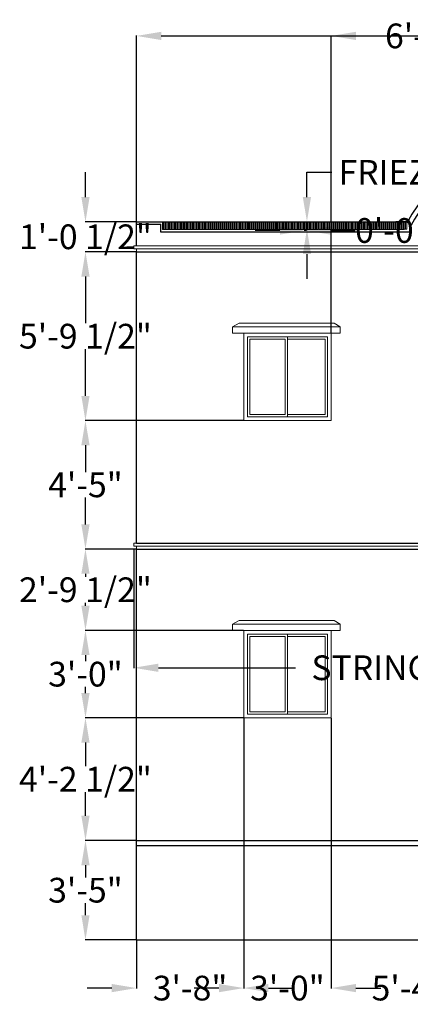
# Model space of a CAD drawing. Units: inches. Extents: x 2393 to 3270, y 740 to 1442.
# Tile 2 of 5: x 2393 to 2554, y 1031 to 1436. Entities that reach past the tile are written whole.
import ezdxf

# ---------------------------------------------------------------- set-up
doc = ezdxf.new("R2010")
doc.units = ezdxf.units.IN
doc.header["$MEASUREMENT"] = 0
for name, color, linetype, lineweight in [('A-ANNO-DIMS', 2, 'Continuous', 18), ('A-ELEV', 7, 'Continuous', 30), ('A-ELEV-TRIM', 8, 'Continuous', 13), ('A-GLAZ', 4, 'Continuous', 18), ('A-ROOF', 7, 'Continuous', 25)]:
    doc.layers.add(name, color=color, linetype=linetype, lineweight=lineweight)
doc.styles.get("Standard").update_dxf_attribs({"font": 'arial.ttf'})
doc.dimstyles.get("Standard").update_dxf_attribs({"dimtxt": 10.18, "dimasz": 10.18, "dimexe": 0.18, "dimexo": 0.0625, "dimgap": 0.09, "dimtad": 0, "dimtih": 1, "dimtoh": 1, "dimdec": 0, "dimzin": 0, "dimdsep": 46, "dimlunit": 3, "dimtxsty": 'Standard', "dimcen": 0.09, "dimadec": 0, "dimazin": 0, "dimtfac": 1, "dimtdec": 0, "dimtofl": 0, "dimtmove": 0, "dimatfit": 3, "dimfxl": 1, "dimtolj": 1, "dimtzin": 0, "dimarcsym": 0})

# ---------------------------------------------------------------- blocks, each defined once
blk = doc.blocks.new('*U4')
for p, q in [((1.5, 1.5), (1.5, 34.5)), ((1.5, 34.5), (18, 34.5)), ((18, 1.5), (18, 34.5)), ((18, 34.5), (34.5, 34.5)), ((34.5, 34.5), (34.5, 1.5)), ((18, 1.5), (1.5, 1.5)), ((34.5, 1.5), (18, 1.5))]:
    blk.add_line(p, q)
blk.add_lwpolyline([(0, 0), (0, 36), (36, 36), (36, 0)], close=True)
for points in [[(17, 33.5), (17, 2.5), (2.5, 2.5), (2.5, 33.5), (17, 33.5)], [(18, 33.5), (33.5, 33.5), (33.5, 2.5), (18, 2.5)]]:
    blk.add_lwpolyline(points)
blk = doc.blocks.new('WIN-HEAD-HOOD-ELEV')
for p, q in [((0, 2.55), (2.7, 4.11)), ((2.7, 4.11), (41.79, 4.11)), ((41.79, 4.11), (44.29, 2.55)), ((0, 0), (0, 2.55)), ((0, 2.55), (44.29, 2.55)), ((0, 0), (4.55, 0)), ((44.29, 0), (40.55, 0)), ((44.29, 2.55), (44.29, 0))]:
    blk.add_line(p, q)
blk = doc.blocks.new('FACADE-STRING-COURSE')
for p, q in [((0.49, 2.4), (0, 2.4)), ((0, 2.4), (0, 1.23)), ((0, 1.23), (1.17, 1.23)), ((0.49, 2.4), (325.84, 2.4)), ((325.84, 1.23), (325.17, 1.23)), ((325.84, 2.4), (325.84, 1.23))]:
    blk.add_line(p, q)
blk.add_lwpolyline([(1.17, 0), (325.17, 0), (325.17, 1.23), (1.17, 1.23)], close=True)
blk = doc.blocks.new('PARAPET-FRIEZE-MODULE')
blk.add_lwpolyline([(0, 3.12), (0.5, 3.12), (0.5, 0), (0, 0)], close=True)
blk = doc.blocks.new('*D38')
at = {"layer": 'A-ANNO-DIMS', "color": 0, "lineweight": -2, "transparency": 16777216}
for p, q in [((2511.53, 1363.37), (2511.53, 1373.55)), ((2511.53, 1373.55), (2521.71, 1373.55)), ((2511.12, 1353.19), (2511.71, 1353.19)), ((2511.12, 1350.06), (2511.71, 1350.06)), ((2511.53, 1339.88), (2511.53, 1329.7))]:
    blk.add_line(p, q, dxfattribs=at)
at = {"layer": 'A-ANNO-DIMS', "color": 0, "transparency": 16777216}
for points in [[(2509.83, 1363.37), (2513.22, 1363.37), (2511.53, 1353.19)], [(2509.83, 1339.88), (2513.22, 1339.88), (2511.53, 1350.06)]]:
    blk.add_solid(points, dxfattribs=at)
at = {"layer": 'Defpoints', "color": 0, "transparency": 16777216}
for p in [(2511.06, 1353.19), (2511.06, 1350.06), (2511.53, 1353.19)]:
    blk.add_point(p, dxfattribs=at)
at = {"layer": 'A-ANNO-DIMS', "color": 0, "transparency": 16777216, "insert": (2579.79, 1373.55), "char_height": 10.18, "attachment_point": 5}
blk.add_mtext('\\A1;FRIEZE 0\'-3" TYP.', dxfattribs=at)
blk = doc.blocks.new('*D39')
at = {"layer": 'A-ANNO-DIMS', "color": 0, "lineweight": -2, "transparency": 16777216}
for p, q in [((2500.38, 1349.6), (2490.2, 1349.6)), ((2510.56, 1350), (2510.56, 1349.42)), ((2511.06, 1350), (2511.06, 1349.42)), ((2521.24, 1349.6), (2531.42, 1349.6))]:
    blk.add_line(p, q, dxfattribs=at)
at = {"layer": 'A-ANNO-DIMS', "color": 0, "transparency": 16777216}
for points in [[(2500.38, 1351.29), (2500.38, 1347.9), (2510.56, 1349.6)], [(2521.24, 1351.29), (2521.24, 1347.9), (2511.06, 1349.6)]]:
    blk.add_solid(points, dxfattribs=at)
at = {"layer": 'Defpoints', "color": 0, "transparency": 16777216}
for p in [(2510.56, 1350.06), (2511.06, 1350.06), (2511.06, 1349.6)]:
    blk.add_point(p, dxfattribs=at)
at = {"layer": 'A-ANNO-DIMS', "color": 0, "transparency": 16777216, "insert": (2574.39, 1349.6), "char_height": 10.18, "attachment_point": 5}
blk.add_mtext('\\A1;0\'-0 1/2" TYP.', dxfattribs=at)
blk = doc.blocks.new('*D40')
at = {"layer": 'A-ANNO-DIMS', "color": 0, "lineweight": -2, "transparency": 16777216}
for p, q in [((2440.26, 1218.37), (2440.26, 1169.38)), ((2766.1, 1218.37), (2766.1, 1169.38)), ((2450.44, 1169.56), (2506.89, 1169.56)), ((2755.92, 1169.56), (2699.46, 1169.56))]:
    blk.add_line(p, q, dxfattribs=at)
at = {"layer": 'A-ANNO-DIMS', "color": 0, "transparency": 16777216}
for points in [[(2450.44, 1171.25), (2450.44, 1167.86), (2440.26, 1169.56)], [(2755.92, 1171.25), (2755.92, 1167.86), (2766.1, 1169.56)]]:
    blk.add_solid(points, dxfattribs=at)
at = {"layer": 'Defpoints', "color": 0, "transparency": 16777216}
for p in [(2440.26, 1218.43), (2766.1, 1218.43), (2766.1, 1169.56)]:
    blk.add_point(p, dxfattribs=at)
at = {"layer": 'A-ANNO-DIMS', "color": 0, "transparency": 16777216, "insert": (2603.18, 1169.56), "char_height": 10.18, "attachment_point": 5}
blk.add_mtext('\\A1;STRING COURSE 27\'-2" TYP.', dxfattribs=at)
blk = doc.blocks.new('*D57')
at = {"layer": 'A-ANNO-DIMS', "color": 0, "lineweight": -2, "transparency": 16777216}
for p, q in [((2441.43, 1353.25), (2441.43, 1429.9)), ((2451.61, 1429.72), (2585.76, 1429.72)), ((2755.25, 1429.72), (2621.09, 1429.72)), ((2765.43, 1353.25), (2765.43, 1429.9))]:
    blk.add_line(p, q, dxfattribs=at)
at = {"layer": 'A-ANNO-DIMS', "color": 0, "transparency": 16777216}
for points in [[(2451.61, 1431.41), (2451.61, 1428.02), (2441.43, 1429.72)], [(2755.25, 1431.41), (2755.25, 1428.02), (2765.43, 1429.72)]]:
    blk.add_solid(points, dxfattribs=at)
at = {"layer": 'Defpoints', "color": 0, "transparency": 16777216}
for p in [(2765.43, 1429.72), (2441.43, 1353.19), (2765.43, 1353.19)]:
    blk.add_point(p, dxfattribs=at)
at = {"layer": 'A-ANNO-DIMS', "color": 0, "transparency": 16777216, "insert": (2603.43, 1429.72), "char_height": 10.18, "attachment_point": 5}
blk.add_mtext('\\A1;27\'-0"', dxfattribs=at)
blk = doc.blocks.new('*D59')
at = {"layer": 'A-ANNO-DIMS', "color": 0, "lineweight": -2, "transparency": 16777216}
for p, q in [((2441.36, 1098.43), (2420.24, 1098.43)), ((2420.42, 1088.25), (2420.42, 1083.26)), ((2420.42, 1067.68), (2420.42, 1072.68)), ((2441.36, 1057.5), (2420.24, 1057.5))]:
    blk.add_line(p, q, dxfattribs=at)
at = {"layer": 'A-ANNO-DIMS', "color": 0, "transparency": 16777216}
for points in [[(2418.73, 1088.25), (2422.12, 1088.25), (2420.42, 1098.43)], [(2418.73, 1067.68), (2422.12, 1067.68), (2420.42, 1057.5)]]:
    blk.add_solid(points, dxfattribs=at)
at = {"layer": 'Defpoints', "color": 0, "transparency": 16777216}
for p in [(2420.42, 1098.43), (2441.43, 1098.43), (2441.43, 1057.5)]:
    blk.add_point(p, dxfattribs=at)
at = {"layer": 'A-ANNO-DIMS', "color": 0, "transparency": 16777216, "insert": (2420.42, 1077.97), "char_height": 10.18, "attachment_point": 5}
blk.add_mtext('\\A1;3\'-5"', dxfattribs=at)
blk = doc.blocks.new('*D60')
at = {"layer": 'A-ANNO-DIMS', "color": 0, "lineweight": -2, "transparency": 16777216}
for p, q in [((2485.45, 1148.93), (2420.24, 1148.93)), ((2420.42, 1138.75), (2420.42, 1129.04)), ((2420.42, 1108.61), (2420.42, 1118.33)), ((2441.36, 1098.43), (2420.24, 1098.43))]:
    blk.add_line(p, q, dxfattribs=at)
at = {"layer": 'A-ANNO-DIMS', "color": 0, "transparency": 16777216}
for points in [[(2418.73, 1138.75), (2422.12, 1138.75), (2420.42, 1148.93)], [(2418.73, 1108.61), (2422.12, 1108.61), (2420.42, 1098.43)]]:
    blk.add_solid(points, dxfattribs=at)
at = {"layer": 'Defpoints', "color": 0, "transparency": 16777216}
for p in [(2420.42, 1148.93), (2485.51, 1148.93), (2441.43, 1098.43)]:
    blk.add_point(p, dxfattribs=at)
at = {"layer": 'A-ANNO-DIMS', "color": 0, "transparency": 16777216, "insert": (2420.42, 1123.68), "char_height": 10.18, "attachment_point": 5}
blk.add_mtext('\\A1;4\'-2 1/2"', dxfattribs=at)
blk = doc.blocks.new('*D61')
at = {"layer": 'A-ANNO-DIMS', "color": 0, "lineweight": -2, "transparency": 16777216}
for p, q in [((2485.45, 1184.93), (2420.24, 1184.93)), ((2420.42, 1174.75), (2420.42, 1172.22)), ((2420.42, 1159.11), (2420.42, 1161.64)), ((2485.45, 1148.93), (2420.24, 1148.93))]:
    blk.add_line(p, q, dxfattribs=at)
at = {"layer": 'A-ANNO-DIMS', "color": 0, "transparency": 16777216}
for points in [[(2418.73, 1174.75), (2422.12, 1174.75), (2420.42, 1184.93)], [(2418.73, 1159.11), (2422.12, 1159.11), (2420.42, 1148.93)]]:
    blk.add_solid(points, dxfattribs=at)
at = {"layer": 'Defpoints', "color": 0, "transparency": 16777216}
for p in [(2420.42, 1184.93), (2485.51, 1184.93), (2485.51, 1148.93)]:
    blk.add_point(p, dxfattribs=at)
at = {"layer": 'A-ANNO-DIMS', "color": 0, "transparency": 16777216, "insert": (2420.42, 1166.93), "char_height": 10.18, "attachment_point": 5}
blk.add_mtext('\\A1;3\'-0"', dxfattribs=at)
blk = doc.blocks.new('*D62')
at = {"layer": 'A-ANNO-DIMS', "color": 0, "lineweight": -2, "transparency": 16777216}
for p, q in [((2441.36, 1218.43), (2420.24, 1218.43)), ((2420.42, 1208.25), (2420.42, 1207.04)), ((2420.42, 1195.11), (2420.42, 1196.33)), ((2485.45, 1184.93), (2420.24, 1184.93))]:
    blk.add_line(p, q, dxfattribs=at)
at = {"layer": 'A-ANNO-DIMS', "color": 0, "transparency": 16777216}
for points in [[(2418.73, 1208.25), (2422.12, 1208.25), (2420.42, 1218.43)], [(2418.73, 1195.11), (2422.12, 1195.11), (2420.42, 1184.93)]]:
    blk.add_solid(points, dxfattribs=at)
at = {"layer": 'Defpoints', "color": 0, "transparency": 16777216}
for p in [(2420.42, 1218.43), (2441.43, 1218.43), (2485.51, 1184.93)]:
    blk.add_point(p, dxfattribs=at)
at = {"layer": 'A-ANNO-DIMS', "color": 0, "transparency": 16777216, "insert": (2420.42, 1201.68), "char_height": 10.18, "attachment_point": 5}
blk.add_mtext('\\A1;2\'-9 1/2"', dxfattribs=at)
blk = doc.blocks.new('*D63')
at = {"layer": 'A-ANNO-DIMS', "color": 0, "lineweight": -2, "transparency": 16777216}
for p, q in [((2485.45, 1271.33), (2420.24, 1271.33)), ((2420.42, 1261.15), (2420.42, 1250.15)), ((2420.42, 1228.61), (2420.42, 1239.61)), ((2441.36, 1218.43), (2420.24, 1218.43))]:
    blk.add_line(p, q, dxfattribs=at)
at = {"layer": 'A-ANNO-DIMS', "color": 0, "transparency": 16777216}
for points in [[(2418.73, 1261.15), (2422.12, 1261.15), (2420.42, 1271.33)], [(2418.73, 1228.61), (2422.12, 1228.61), (2420.42, 1218.43)]]:
    blk.add_solid(points, dxfattribs=at)
at = {"layer": 'Defpoints', "color": 0, "transparency": 16777216}
for p in [(2420.42, 1271.33), (2485.51, 1271.33), (2441.43, 1218.43)]:
    blk.add_point(p, dxfattribs=at)
at = {"layer": 'A-ANNO-DIMS', "color": 0, "transparency": 16777216, "insert": (2420.42, 1244.88), "char_height": 10.18, "attachment_point": 5}
blk.add_mtext('\\A1;4\'-5"', dxfattribs=at)
blk = doc.blocks.new('*D64')
at = {"layer": 'A-ANNO-DIMS', "color": 0, "lineweight": -2, "transparency": 16777216}
for p, q in [((2441.36, 1340.83), (2420.24, 1340.83)), ((2420.42, 1330.65), (2420.42, 1311.43)), ((2420.42, 1281.51), (2420.42, 1300.72)), ((2485.45, 1271.33), (2420.24, 1271.33))]:
    blk.add_line(p, q, dxfattribs=at)
at = {"layer": 'A-ANNO-DIMS', "color": 0, "transparency": 16777216}
for points in [[(2418.73, 1330.65), (2422.12, 1330.65), (2420.42, 1340.83)], [(2418.73, 1281.51), (2422.12, 1281.51), (2420.42, 1271.33)]]:
    blk.add_solid(points, dxfattribs=at)
at = {"layer": 'Defpoints', "color": 0, "transparency": 16777216}
for p in [(2420.42, 1340.83), (2441.43, 1340.83), (2485.51, 1271.33)]:
    blk.add_point(p, dxfattribs=at)
at = {"layer": 'A-ANNO-DIMS', "color": 0, "transparency": 16777216, "insert": (2420.42, 1306.08), "char_height": 10.18, "attachment_point": 5}
blk.add_mtext('\\A1;5\'-9 1/2"', dxfattribs=at)
blk = doc.blocks.new('*D65')
at = {"layer": 'A-ANNO-DIMS', "color": 0, "lineweight": -2, "transparency": 16777216}
for p, q in [((2420.42, 1363.37), (2420.42, 1373.55)), ((2441.36, 1353.19), (2420.24, 1353.19)), ((2441.36, 1340.83), (2420.24, 1340.83)), ((2420.42, 1330.65), (2420.42, 1320.47))]:
    blk.add_line(p, q, dxfattribs=at)
at = {"layer": 'A-ANNO-DIMS', "color": 0, "transparency": 16777216}
for points in [[(2418.73, 1363.37), (2422.12, 1363.37), (2420.42, 1353.19)], [(2418.73, 1330.65), (2422.12, 1330.65), (2420.42, 1340.83)]]:
    blk.add_solid(points, dxfattribs=at)
at = {"layer": 'Defpoints', "color": 0, "transparency": 16777216}
for p in [(2420.42, 1353.19), (2441.43, 1353.19), (2441.43, 1340.83)]:
    blk.add_point(p, dxfattribs=at)
at = {"layer": 'A-ANNO-DIMS', "color": 0, "transparency": 16777216, "insert": (2420.42, 1347.01), "char_height": 10.18, "attachment_point": 5}
blk.add_mtext('\\A1;1\'-0 1/2"', dxfattribs=at)
blk = doc.blocks.new('*D67')
at = {"layer": 'A-ANNO-DIMS', "color": 0, "lineweight": -2, "transparency": 16777216}
for p, q in [((2485.51, 1148.87), (2485.51, 1037.49)), ((2441.43, 1057.44), (2441.43, 1037.49)), ((2431.25, 1037.67), (2421.07, 1037.67)), ((2495.69, 1037.67), (2505.87, 1037.67))]:
    blk.add_line(p, q, dxfattribs=at)
at = {"layer": 'A-ANNO-DIMS', "color": 0, "transparency": 16777216}
for points in [[(2431.25, 1039.37), (2431.25, 1035.97), (2441.43, 1037.67)], [(2495.69, 1039.37), (2495.69, 1035.97), (2485.51, 1037.67)]]:
    blk.add_solid(points, dxfattribs=at)
at = {"layer": 'Defpoints', "color": 0, "transparency": 16777216}
for p in [(2485.51, 1148.93), (2441.43, 1057.5), (2485.51, 1037.67)]:
    blk.add_point(p, dxfattribs=at)
at = {"layer": 'A-ANNO-DIMS', "color": 0, "transparency": 16777216, "insert": (2463.47, 1037.67), "char_height": 10.18, "attachment_point": 5}
blk.add_mtext('\\A1;3\'-8"', dxfattribs=at)
blk = doc.blocks.new('*D68')
at = {"layer": 'A-ANNO-DIMS', "color": 0, "lineweight": -2, "transparency": 16777216}
for p, q in [((2485.51, 1148.87), (2485.51, 1037.49)), ((2521.51, 1148.87), (2521.51, 1037.49)), ((2475.33, 1037.67), (2465.15, 1037.67)), ((2531.69, 1037.67), (2541.87, 1037.67))]:
    blk.add_line(p, q, dxfattribs=at)
at = {"layer": 'A-ANNO-DIMS', "color": 0, "transparency": 16777216}
for points in [[(2475.33, 1039.37), (2475.33, 1035.97), (2485.51, 1037.67)], [(2531.69, 1039.37), (2531.69, 1035.97), (2521.51, 1037.67)]]:
    blk.add_solid(points, dxfattribs=at)
at = {"layer": 'Defpoints', "color": 0, "transparency": 16777216}
for p in [(2485.51, 1148.93), (2521.51, 1148.93), (2521.51, 1037.67)]:
    blk.add_point(p, dxfattribs=at)
at = {"layer": 'A-ANNO-DIMS', "color": 0, "transparency": 16777216, "insert": (2503.51, 1037.67), "char_height": 10.18, "attachment_point": 5}
blk.add_mtext('\\A1;3\'-0"', dxfattribs=at)
blk = doc.blocks.new('*D69')
at = {"layer": 'A-ANNO-DIMS', "color": 0, "lineweight": -2, "transparency": 16777216}
for p, q in [((2521.51, 1148.87), (2521.51, 1037.49)), ((2585.43, 1098.37), (2585.43, 1037.49)), ((2531.69, 1037.67), (2539.85, 1037.67)), ((2575.25, 1037.67), (2567.09, 1037.67))]:
    blk.add_line(p, q, dxfattribs=at)
at = {"layer": 'A-ANNO-DIMS', "color": 0, "transparency": 16777216}
for points in [[(2531.69, 1039.37), (2531.69, 1035.97), (2521.51, 1037.67)], [(2575.25, 1039.37), (2575.25, 1035.97), (2585.43, 1037.67)]]:
    blk.add_solid(points, dxfattribs=at)
at = {"layer": 'Defpoints', "color": 0, "transparency": 16777216}
for p in [(2521.51, 1148.93), (2585.43, 1098.43), (2585.43, 1037.67)]:
    blk.add_point(p, dxfattribs=at)
at = {"layer": 'A-ANNO-DIMS', "color": 0, "transparency": 16777216, "insert": (2553.47, 1037.67), "char_height": 10.18, "attachment_point": 5}
blk.add_mtext('\\A1;5\'-4"', dxfattribs=at)
blk = doc.blocks.new('*D72')
at = {"layer": 'A-ANNO-DIMS', "color": 0, "lineweight": -2, "transparency": 16777216}
for p, q in [((2521.51, 1307.39), (2521.51, 1429.9)), ((2531.69, 1429.72), (2545.34, 1429.72)), ((2586.29, 1429.72), (2572.64, 1429.72)), ((2596.47, 1307.39), (2596.47, 1429.9))]:
    blk.add_line(p, q, dxfattribs=at)
at = {"layer": 'A-ANNO-DIMS', "color": 0, "transparency": 16777216}
for points in [[(2531.69, 1431.41), (2531.69, 1428.02), (2521.51, 1429.72)], [(2586.29, 1431.41), (2586.29, 1428.02), (2596.47, 1429.72)]]:
    blk.add_solid(points, dxfattribs=at)
at = {"layer": 'Defpoints', "color": 0, "transparency": 16777216}
for p in [(2596.47, 1429.72), (2521.51, 1307.33), (2596.47, 1307.33)]:
    blk.add_point(p, dxfattribs=at)
at = {"layer": 'A-ANNO-DIMS', "color": 0, "transparency": 16777216, "insert": (2558.99, 1429.72), "char_height": 10.18, "attachment_point": 5}
blk.add_mtext('\\A1;6\'-3"', dxfattribs=at)

msp = doc.modelspace()

# ---------------------------------------------------------------- linework, layer by layer
at = {"layer": 'A-ELEV'}
for p, q in [((2441.43, 1220.83), (2441.43, 1340.83)), ((2441.43, 1340.83), (2765.43, 1340.83)), ((2441.43, 1220.83), (2765.43, 1220.83)), ((2441.43, 1098.43), (2441.43, 1218.43)), ((2441.43, 1218.43), (2765.43, 1218.43)), ((2441.43, 1057.5), (2441.43, 1098.43)), ((2441.43, 1098.43), (2765.43, 1098.43)), ((2441.43, 1096.43), (2765.43, 1096.43)), ((2441.43, 1057.5), (2765.43, 1057.5))]:
    msp.add_line(p, q, dxfattribs=at)
at = {"layer": 'A-ELEV-TRIM'}
for points in [[(2551.09, 1350.37), (2551.09, 1353.19)], [(2551.59, 1353.19), (2551.59, 1350.37)], [(2552.08, 1353.19), (2552.08, 1350.15), (2551.59, 1350.15), (2551.59, 1353.19)], [(2551.59, 1350.37), (2551.59, 1353.19)], [(2552.08, 1353.19), (2552.08, 1350.37)], [(2552.58, 1352.57), (2552.58, 1350.15), (2552.08, 1350.15), (2552.08, 1353.19)], [(2552.08, 1350.37), (2552.08, 1353.19)], [(2552.58, 1353.19), (2552.58, 1353.19)], [(2552.58, 1353.19), (2552.58, 1353.19)], [(2552.58, 1352.57), (2552.58, 1350.37)]]:
    msp.add_lwpolyline(points, dxfattribs=at)
at = {"layer": 'A-ROOF'}
for p, q in [((2441.43, 1343.22), (2441.43, 1353.19)), ((2441.43, 1353.19), (2498.71, 1353.19)), ((2441.43, 1352.17), (2451.47, 1352.17)), ((2451.47, 1348.89), (2451.47, 1352.17)), ((2498.71, 1353.19), (2552.91, 1353.19)), ((2552.91, 1353.19), (2548.05, 1353.19)), ((2553.79, 1350.55), (2553.79, 1348.89)), ((2553.79, 1348.89), (2451.47, 1348.89))]:
    msp.add_line(p, q, dxfattribs=at)
for radius, start, end in [(59.93, 24.2594, 152.1815), (57.93, 24.2995, 153.3937)]:
    msp.add_arc((2605.58, 1324.61), radius, start, end, dxfattribs=at)

# ---------------------------------------------------------------- block references
at = {"layer": 'A-ELEV-TRIM'}
for name, p in [('PARAPET-FRIEZE-MODULE', (2452.05, 1350.06)), ('PARAPET-FRIEZE-MODULE', (2452.54, 1350.06)), ('PARAPET-FRIEZE-MODULE', (2453.04, 1350.06)), ('PARAPET-FRIEZE-MODULE', (2453.53, 1350.06)), ('PARAPET-FRIEZE-MODULE', (2454.03, 1350.06)), ('PARAPET-FRIEZE-MODULE', (2454.52, 1350.06)), ('PARAPET-FRIEZE-MODULE', (2455.02, 1350.06)), ('PARAPET-FRIEZE-MODULE', (2455.51, 1350.06)), ('PARAPET-FRIEZE-MODULE', (2456.01, 1350.06)), ('PARAPET-FRIEZE-MODULE', (2456.5, 1350.06)), ('PARAPET-FRIEZE-MODULE', (2457, 1350.06)), ('PARAPET-FRIEZE-MODULE', (2457.49, 1350.06)), ('PARAPET-FRIEZE-MODULE', (2457.98, 1350.06)), ('PARAPET-FRIEZE-MODULE', (2458.48, 1350.06)), ('PARAPET-FRIEZE-MODULE', (2458.97, 1350.06)), ('PARAPET-FRIEZE-MODULE', (2459.47, 1350.06)), ('PARAPET-FRIEZE-MODULE', (2459.96, 1350.06)), ('PARAPET-FRIEZE-MODULE', (2460.46, 1350.06)), ('PARAPET-FRIEZE-MODULE', (2460.95, 1350.06)), ('PARAPET-FRIEZE-MODULE', (2461.45, 1350.06)), ('PARAPET-FRIEZE-MODULE', (2461.94, 1350.06)), ('PARAPET-FRIEZE-MODULE', (2462.44, 1350.06)), ('PARAPET-FRIEZE-MODULE', (2462.93, 1350.06)), ('PARAPET-FRIEZE-MODULE', (2463.43, 1350.06)), ('PARAPET-FRIEZE-MODULE', (2463.92, 1350.06)), ('PARAPET-FRIEZE-MODULE', (2464.42, 1350.06)), ('PARAPET-FRIEZE-MODULE', (2464.91, 1350.06)), ('PARAPET-FRIEZE-MODULE', (2465.41, 1350.06)), ('PARAPET-FRIEZE-MODULE', (2465.9, 1350.06)), ('PARAPET-FRIEZE-MODULE', (2466.4, 1350.06)), ('PARAPET-FRIEZE-MODULE', (2466.89, 1350.06)), ('PARAPET-FRIEZE-MODULE', (2467.39, 1350.06)), ('PARAPET-FRIEZE-MODULE', (2467.88, 1350.06)), ('PARAPET-FRIEZE-MODULE', (2468.38, 1350.06)), ('PARAPET-FRIEZE-MODULE', (2468.87, 1350.06)), ('PARAPET-FRIEZE-MODULE', (2469.37, 1350.06)), ('PARAPET-FRIEZE-MODULE', (2469.86, 1350.06)), ('PARAPET-FRIEZE-MODULE', (2470.36, 1350.06)), ('PARAPET-FRIEZE-MODULE', (2470.85, 1350.06)), ('PARAPET-FRIEZE-MODULE', (2471.35, 1350.06)), ('PARAPET-FRIEZE-MODULE', (2471.84, 1350.06)), ('PARAPET-FRIEZE-MODULE', (2472.34, 1350.06)), ('PARAPET-FRIEZE-MODULE', (2472.83, 1350.06)), ('PARAPET-FRIEZE-MODULE', (2473.32, 1350.06)), ('PARAPET-FRIEZE-MODULE', (2473.82, 1350.06)), ('PARAPET-FRIEZE-MODULE', (2474.31, 1350.06)), ('PARAPET-FRIEZE-MODULE', (2474.81, 1350.06)), ('PARAPET-FRIEZE-MODULE', (2475.3, 1350.06)), ('PARAPET-FRIEZE-MODULE', (2475.8, 1350.06)), ('PARAPET-FRIEZE-MODULE', (2476.29, 1350.06)), ('PARAPET-FRIEZE-MODULE', (2476.79, 1350.06)), ('PARAPET-FRIEZE-MODULE', (2477.28, 1350.06)), ('PARAPET-FRIEZE-MODULE', (2477.78, 1350.06)), ('PARAPET-FRIEZE-MODULE', (2478.27, 1350.06)), ('PARAPET-FRIEZE-MODULE', (2478.77, 1350.06)), ('PARAPET-FRIEZE-MODULE', (2479.26, 1350.06)), ('PARAPET-FRIEZE-MODULE', (2479.76, 1350.06)), ('PARAPET-FRIEZE-MODULE', (2480.25, 1350.06)), ('PARAPET-FRIEZE-MODULE', (2480.75, 1350.06)), ('PARAPET-FRIEZE-MODULE', (2481.24, 1350.06)), ('PARAPET-FRIEZE-MODULE', (2481.74, 1350.06)), ('PARAPET-FRIEZE-MODULE', (2482.23, 1350.06)), ('PARAPET-FRIEZE-MODULE', (2482.73, 1350.06)), ('PARAPET-FRIEZE-MODULE', (2483.22, 1350.06)), ('PARAPET-FRIEZE-MODULE', (2483.72, 1350.06)), ('PARAPET-FRIEZE-MODULE', (2484.21, 1350.06)), ('PARAPET-FRIEZE-MODULE', (2484.71, 1350.06)), ('PARAPET-FRIEZE-MODULE', (2485.2, 1350.06)), ('PARAPET-FRIEZE-MODULE', (2485.7, 1350.06)), ('PARAPET-FRIEZE-MODULE', (2486.56, 1350.06)), ('PARAPET-FRIEZE-MODULE', (2487.06, 1350.06)), ('PARAPET-FRIEZE-MODULE', (2487.55, 1350.06)), ('PARAPET-FRIEZE-MODULE', (2488.05, 1350.06)), ('PARAPET-FRIEZE-MODULE', (2488.54, 1350.06)), ('PARAPET-FRIEZE-MODULE', (2489.04, 1350.06)), ('PARAPET-FRIEZE-MODULE', (2489.53, 1350.06)), ('PARAPET-FRIEZE-MODULE', (2490.03, 1350.06)), ('PARAPET-FRIEZE-MODULE', (2490.52, 1350.06)), ('PARAPET-FRIEZE-MODULE', (2491.02, 1350.06)), ('PARAPET-FRIEZE-MODULE', (2491.51, 1350.06)), ('PARAPET-FRIEZE-MODULE', (2492.01, 1350.06)), ('PARAPET-FRIEZE-MODULE', (2492.5, 1350.06)), ('PARAPET-FRIEZE-MODULE', (2493, 1350.06)), ('PARAPET-FRIEZE-MODULE', (2493.49, 1350.06)), ('PARAPET-FRIEZE-MODULE', (2493.99, 1350.06)), ('PARAPET-FRIEZE-MODULE', (2494.48, 1350.06)), ('PARAPET-FRIEZE-MODULE', (2494.98, 1350.06)), ('PARAPET-FRIEZE-MODULE', (2495.47, 1350.06)), ('PARAPET-FRIEZE-MODULE', (2495.97, 1350.06)), ('PARAPET-FRIEZE-MODULE', (2496.46, 1350.06)), ('PARAPET-FRIEZE-MODULE', (2496.95, 1350.06)), ('PARAPET-FRIEZE-MODULE', (2497.45, 1350.06)), ('PARAPET-FRIEZE-MODULE', (2497.94, 1350.06)), ('PARAPET-FRIEZE-MODULE', (2498.44, 1350.06)), ('PARAPET-FRIEZE-MODULE', (2498.93, 1350.06)), ('PARAPET-FRIEZE-MODULE', (2499.43, 1350.06)), ('PARAPET-FRIEZE-MODULE', (2499.92, 1350.06)), ('PARAPET-FRIEZE-MODULE', (2500.42, 1350.06)), ('PARAPET-FRIEZE-MODULE', (2500.91, 1350.06)), ('PARAPET-FRIEZE-MODULE', (2501.41, 1350.06)), ('PARAPET-FRIEZE-MODULE', (2501.66, 1350.06)), ('PARAPET-FRIEZE-MODULE', (2502.15, 1350.06)), ('PARAPET-FRIEZE-MODULE', (2502.65, 1350.06)), ('PARAPET-FRIEZE-MODULE', (2503.14, 1350.06)), ('PARAPET-FRIEZE-MODULE', (2503.64, 1350.06)), ('PARAPET-FRIEZE-MODULE', (2504.13, 1350.06)), ('PARAPET-FRIEZE-MODULE', (2504.62, 1350.06)), ('PARAPET-FRIEZE-MODULE', (2505.12, 1350.06)), ('PARAPET-FRIEZE-MODULE', (2505.61, 1350.06)), ('PARAPET-FRIEZE-MODULE', (2506.11, 1350.06)), ('PARAPET-FRIEZE-MODULE', (2506.6, 1350.06)), ('PARAPET-FRIEZE-MODULE', (2507.1, 1350.06)), ('PARAPET-FRIEZE-MODULE', (2507.59, 1350.06)), ('PARAPET-FRIEZE-MODULE', (2508.09, 1350.06)), ('PARAPET-FRIEZE-MODULE', (2508.58, 1350.06)), ('PARAPET-FRIEZE-MODULE', (2509.08, 1350.06)), ('PARAPET-FRIEZE-MODULE', (2509.57, 1350.06)), ('PARAPET-FRIEZE-MODULE', (2510.07, 1350.06)), ('PARAPET-FRIEZE-MODULE', (2510.56, 1350.06)), ('PARAPET-FRIEZE-MODULE', (2511.06, 1350.06)), ('PARAPET-FRIEZE-MODULE', (2511.55, 1350.06)), ('PARAPET-FRIEZE-MODULE', (2512.05, 1350.06)), ('PARAPET-FRIEZE-MODULE', (2512.54, 1350.06)), ('PARAPET-FRIEZE-MODULE', (2513.04, 1350.06)), ('PARAPET-FRIEZE-MODULE', (2513.53, 1350.06)), ('PARAPET-FRIEZE-MODULE', (2514.03, 1350.06)), ('PARAPET-FRIEZE-MODULE', (2514.52, 1350.06)), ('PARAPET-FRIEZE-MODULE', (2515.02, 1350.06)), ('PARAPET-FRIEZE-MODULE', (2515.51, 1350.06)), ('PARAPET-FRIEZE-MODULE', (2516.34, 1350.06)), ('PARAPET-FRIEZE-MODULE', (2516.84, 1350.06)), ('PARAPET-FRIEZE-MODULE', (2517.33, 1350.06)), ('PARAPET-FRIEZE-MODULE', (2517.83, 1350.06)), ('PARAPET-FRIEZE-MODULE', (2518.32, 1350.06)), ('PARAPET-FRIEZE-MODULE', (2518.82, 1350.06)), ('PARAPET-FRIEZE-MODULE', (2519.31, 1350.06)), ('PARAPET-FRIEZE-MODULE', (2519.81, 1350.06)), ('PARAPET-FRIEZE-MODULE', (2520.3, 1350.06)), ('PARAPET-FRIEZE-MODULE', (2520.8, 1350.06)), ('PARAPET-FRIEZE-MODULE', (2521.29, 1350.06)), ('PARAPET-FRIEZE-MODULE', (2521.79, 1350.06)), ('PARAPET-FRIEZE-MODULE', (2522.28, 1350.06)), ('PARAPET-FRIEZE-MODULE', (2522.78, 1350.06)), ('PARAPET-FRIEZE-MODULE', (2523.27, 1350.06)), ('PARAPET-FRIEZE-MODULE', (2523.77, 1350.06)), ('PARAPET-FRIEZE-MODULE', (2524.26, 1350.06)), ('PARAPET-FRIEZE-MODULE', (2524.76, 1350.06)), ('PARAPET-FRIEZE-MODULE', (2525.25, 1350.06)), ('PARAPET-FRIEZE-MODULE', (2525.75, 1350.06)), ('PARAPET-FRIEZE-MODULE', (2526.24, 1350.06)), ('PARAPET-FRIEZE-MODULE', (2526.85, 1350.06)), ('PARAPET-FRIEZE-MODULE', (2527.34, 1350.06)), ('PARAPET-FRIEZE-MODULE', (2527.84, 1350.06)), ('PARAPET-FRIEZE-MODULE', (2528.33, 1350.06)), ('PARAPET-FRIEZE-MODULE', (2528.83, 1350.06)), ('PARAPET-FRIEZE-MODULE', (2529.32, 1350.06)), ('PARAPET-FRIEZE-MODULE', (2529.82, 1350.06)), ('PARAPET-FRIEZE-MODULE', (2530.31, 1350.06)), ('PARAPET-FRIEZE-MODULE', (2530.81, 1350.06)), ('PARAPET-FRIEZE-MODULE', (2531.3, 1350.06)), ('PARAPET-FRIEZE-MODULE', (2531.8, 1350.06)), ('PARAPET-FRIEZE-MODULE', (2532.29, 1350.06)), ('PARAPET-FRIEZE-MODULE', (2532.78, 1350.06)), ('PARAPET-FRIEZE-MODULE', (2533.28, 1350.06)), ('PARAPET-FRIEZE-MODULE', (2533.77, 1350.06)), ('PARAPET-FRIEZE-MODULE', (2534.27, 1350.06)), ('PARAPET-FRIEZE-MODULE', (2534.76, 1350.06)), ('PARAPET-FRIEZE-MODULE', (2535.26, 1350.06)), ('PARAPET-FRIEZE-MODULE', (2535.75, 1350.06)), ('PARAPET-FRIEZE-MODULE', (2536.25, 1350.06)), ('PARAPET-FRIEZE-MODULE', (2536.74, 1350.06)), ('PARAPET-FRIEZE-MODULE', (2537.24, 1350.06)), ('PARAPET-FRIEZE-MODULE', (2537.73, 1350.06)), ('PARAPET-FRIEZE-MODULE', (2538.23, 1350.06)), ('PARAPET-FRIEZE-MODULE', (2538.72, 1350.06)), ('PARAPET-FRIEZE-MODULE', (2539.22, 1350.06)), ('PARAPET-FRIEZE-MODULE', (2539.71, 1350.06)), ('PARAPET-FRIEZE-MODULE', (2540.21, 1350.06)), ('PARAPET-FRIEZE-MODULE', (2540.7, 1350.06)), ('PARAPET-FRIEZE-MODULE', (2541.2, 1350.06)), ('PARAPET-FRIEZE-MODULE', (2541.69, 1350.06)), ('PARAPET-FRIEZE-MODULE', (2542.19, 1350.06)), ('PARAPET-FRIEZE-MODULE', (2542.68, 1350.06)), ('PARAPET-FRIEZE-MODULE', (2543.18, 1350.06)), ('PARAPET-FRIEZE-MODULE', (2543.67, 1350.06)), ('PARAPET-FRIEZE-MODULE', (2544.17, 1350.06)), ('PARAPET-FRIEZE-MODULE', (2544.66, 1350.06)), ('PARAPET-FRIEZE-MODULE', (2545.16, 1350.06)), ('PARAPET-FRIEZE-MODULE', (2545.65, 1350.06)), ('PARAPET-FRIEZE-MODULE', (2546.15, 1350.06)), ('PARAPET-FRIEZE-MODULE', (2546.64, 1350.06)), ('PARAPET-FRIEZE-MODULE', (2547.13, 1350.06)), ('PARAPET-FRIEZE-MODULE', (2547.63, 1350.06)), ('PARAPET-FRIEZE-MODULE', (2548.12, 1350.06)), ('PARAPET-FRIEZE-MODULE', (2548.62, 1350.06)), ('PARAPET-FRIEZE-MODULE', (2549.11, 1350.06)), ('PARAPET-FRIEZE-MODULE', (2549.61, 1350.06)), ('PARAPET-FRIEZE-MODULE', (2550.1, 1350.06)), ('PARAPET-FRIEZE-MODULE', (2550.6, 1350.06)), ('PARAPET-FRIEZE-MODULE', (2551.09, 1350.06)), ('FACADE-STRING-COURSE', (2440.26, 1340.83)), ('WIN-HEAD-HOOD-ELEV', (2480.95, 1307.33)), ('FACADE-STRING-COURSE', (2440.26, 1218.43)), ('WIN-HEAD-HOOD-ELEV', (2480.95, 1184.93))]:
    msp.add_blockref(name, p, dxfattribs=at)
at = {"layer": 'A-GLAZ'}
for p in [(2485.51, 1271.33), (2485.51, 1148.93)]:
    msp.add_blockref('*U4', p, dxfattribs=at)

# ---------------------------------------------------------------- dimensions: what is measured, and where the dimension line sits
at = {"layer": 'A-ANNO-DIMS'}
for base, p1, p2, picture, middle in [((2765.43, 1429.72), (2441.43, 1353.19), (2765.43, 1353.19), '*D57', (2603.43, 1429.72)), ((2596.47, 1429.72), (2521.51, 1307.33), (2596.47, 1307.33), '*D72', (2558.99, 1429.72)), ((2485.51, 1037.67), (2441.43, 1057.5), (2485.51, 1148.93), '*D67', (2463.47, 1037.67)), ((2521.51, 1037.67), (2485.51, 1148.93), (2521.51, 1148.93), '*D68', (2503.51, 1037.67)), ((2585.43, 1037.67), (2521.51, 1148.93), (2585.43, 1098.43), '*D69', (2553.47, 1037.67))]:
    dim = msp.add_linear_dim(base=base, p1=p1, p2=p2, dimstyle='Standard', override={"dimdec": 1, "dimlfac": 1, "dimrnd": 0, "dimzin": 1, "dimdsep": 46, "dimlunit": 4, "dimfrac": 2}, dxfattribs=at)
    dim.commit()
    dim.dimension.update_dxf_attribs({"geometry": picture, "text_midpoint": middle})
dim = msp.add_linear_dim(base=(2511.53, 1353.19), p1=(2511.06, 1350.06), p2=(2511.06, 1353.19), angle=90, text='FRIEZE <> TYP.', dimstyle='Standard', override={"dimdec": 1, "dimlfac": 1, "dimrnd": 0, "dimzin": 1, "dimdsep": 46, "dimlunit": 4, "dimfrac": 2}, dxfattribs=at)
dim.commit()
dim.dimension.update_dxf_attribs({"geometry": '*D38', "text_midpoint": (2579.79, 1373.55)})
for base, p1, p2, picture, middle in [((2420.42, 1353.19), (2441.43, 1340.83), (2441.43, 1353.19), '*D65', (2420.42, 1347.01)), ((2420.42, 1340.83), (2485.51, 1271.33), (2441.43, 1340.83), '*D64', (2420.42, 1306.08)), ((2420.42, 1271.33), (2441.43, 1218.43), (2485.51, 1271.33), '*D63', (2420.42, 1244.88)), ((2420.42, 1218.43), (2485.51, 1184.93), (2441.43, 1218.43), '*D62', (2420.42, 1201.68)), ((2420.42, 1184.93), (2485.51, 1148.93), (2485.51, 1184.93), '*D61', (2420.42, 1166.93)), ((2420.42, 1148.93), (2441.43, 1098.43), (2485.51, 1148.93), '*D60', (2420.42, 1123.68)), ((2420.42, 1098.43), (2441.43, 1057.5), (2441.43, 1098.43), '*D59', (2420.42, 1077.97))]:
    dim = msp.add_linear_dim(base=base, p1=p1, p2=p2, angle=90, dimstyle='Standard', override={"dimdec": 1, "dimlfac": 1, "dimrnd": 0, "dimzin": 1, "dimdsep": 46, "dimlunit": 4, "dimfrac": 2}, dxfattribs=at)
    dim.commit()
    dim.dimension.update_dxf_attribs({"geometry": picture, "text_midpoint": middle})
for base, p1, p2, text, picture, middle in [((2511.06, 1349.6), (2510.56, 1350.06), (2511.06, 1350.06), '<> TYP.', '*D39', (2574.39, 1349.6)), ((2766.1, 1169.56), (2440.26, 1218.43), (2766.1, 1218.43), 'STRING COURSE <> TYP.', '*D40', (2603.18, 1169.56))]:
    dim = msp.add_linear_dim(base=base, p1=p1, p2=p2, text=text, dimstyle='Standard', override={"dimdec": 1, "dimlfac": 1, "dimrnd": 0, "dimzin": 1, "dimdsep": 46, "dimlunit": 4, "dimfrac": 2}, dxfattribs=at)
    dim.commit()
    dim.dimension.update_dxf_attribs({"geometry": picture, "text_midpoint": middle})

doc.saveas('drawing.dxf')
